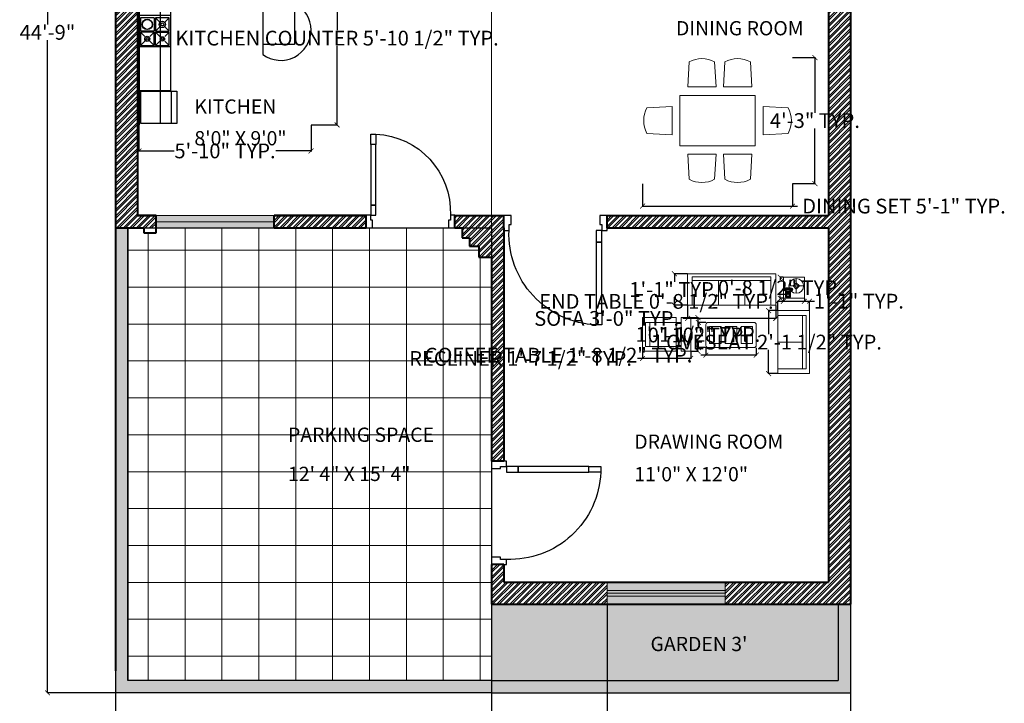
# Model space of a CAD drawing. Units: inches. Extents: x 528 to 2520, y -151 to 1354.
# Tile 29 of 41: x 2119 to 2520, y 357 to 635. Entities that reach past the tile are written whole.
import ezdxf

# ---------------------------------------------------------------- set-up
doc = ezdxf.new("R2010")
doc.units = ezdxf.units.IN
doc.header["$MEASUREMENT"] = 0
for name, color, linetype, lineweight in [('A-ANNO-DIMS', 2, 'Continuous', 18), ('A-AREA-IDEN', 7, 'Continuous', 18), ('A-Door', 150, 'Continuous', 25), ('A-ELEV-PROJ', 8, 'Continuous', 13), ('A-FLOR-CASE', 11, 'Continuous', 20), ('A-FLOR-PATT', 7, 'Continuous', 13), ('A-FURN', 8, 'Continuous', 18), ('A-SITE-EDGE', 7, 'Continuous', 25), ('A-SITE-PATT', 7, 'Continuous', 13), ('A-WALL-PATT', 6, 'Continuous', 13), ('walls', 7, 'Continuous', 40), ('WINDOWS', 2, 'Continuous', 20)]:
    doc.layers.add(name, color=color, linetype=linetype, lineweight=lineweight)
doc.layers.add('A-GLAZ-PATT', color=152, linetype='Continuous', lineweight=13, true_color=0x2776bb)
doc.layers.add('L-PLNT-PATT', color=85, linetype='Continuous', lineweight=13, true_color=0x58ba48)
for name, color, linetype in [('ESYA', 11, 'Continuous'), ('NT', 1, 'Continuous'), ('TEFRIS', 11, 'Continuous')]:
    doc.layers.add(name, color=color, linetype=linetype)
doc.styles.get("Standard").update_dxf_attribs({"font": 'arial.ttf'})
doc.dimstyles.get("Standard").update_dxf_attribs({"dimtxt": 6, "dimasz": 2, "dimexe": 0.18, "dimexo": 0.0625, "dimgap": 0.09, "dimtad": 0, "dimtih": 1, "dimtoh": 1, "dimdec": 1, "dimzin": 0, "dimdsep": 46, "dimlunit": 3, "dimtxsty": 'Standard', "dimblk": 'ARCHTICK', "dimcen": 0.09, "dimadec": 0, "dimazin": 0, "dimtfac": 1, "dimtdec": 1, "dimtofl": 0, "dimtmove": 0, "dimatfit": 3, "dimfxl": 1, "dimtolj": 1, "dimtzin": 0, "dimarcsym": 0})

# ---------------------------------------------------------------- blocks, each defined once
blk = doc.blocks.new('A$C7DB75F4D')
at = {"layer": 'A-Door'}
for points in [[(625, 740), (625, 660), (665, 660), (665, 740)], [(625, 180), (625, 660), (665, 660), (665, 180)], [(625, 100), (625, 180), (665, 180), (665, 100)], [(35, 100), (35, 60), (50, 60), (50, 50), (50, 0), (0, 0), (0, 100)], [(665, 100), (700, 100), (700, 0), (650, 0), (650, 50), (650, 60), (665, 60)]]:
    blk.add_lwpolyline(points, close=True, dxfattribs=at)
at = {"layer": 'NT'}
blk.add_arc((650, 125), 615.5, 92.32782, 182.32782, dxfattribs=at)
blk = doc.blocks.new('AR365L')
blk.add_line((0, 0.1), (0.61, 0.1))
blk.add_lwpolyline([(0, 0), (0, 0.68), (0.61, 0.68), (0.61, 0)], close=True)
blk = doc.blocks.new('FIRIN1')
at = {"layer": 'ESYA'}
for p, q in [((0.288, -0.05), (0.288, -0.301)), ((0.398, -0.132), (0.312, -0.05)), ((0.575, -0.05), (0.489, -0.132)), ((0.288, -0.301), (0.025, -0.301)), ((0.025, -0.324), (0.111, -0.406)), ((0.202, -0.406), (0.288, -0.324)), ((0.398, -0.219), (0.312, -0.301)), ((0.398, -0.406), (0.312, -0.324)), ((0.575, -0.301), (0.489, -0.219)), ((0.575, -0.324), (0.489, -0.406)), ((0.025, -0.575), (0.111, -0.493)), ((0.202, -0.493), (0.288, -0.575)), ((0.398, -0.493), (0.312, -0.575)), ((0.575, -0.575), (0.489, -0.493))]:
    blk.add_line(p, q, dxfattribs=at)
blk.add_lwpolyline([(0, 0), (0.6, 0), (0.6, -0.6), (0, -0.6)], close=True, dxfattribs=at)
for points in [[(0.288, -0.05), (0.025, -0.05), (0.025, -0.301)], [(0.312, -0.05), (0.312, -0.301), (0.575, -0.301)], [(0.575, -0.301), (0.575, -0.05), (0.312, -0.05)], [(0.288, -0.575), (0.288, -0.324), (0.025, -0.324)], [(0.025, -0.324), (0.025, -0.575)], [(0.312, -0.575), (0.312, -0.324), (0.575, -0.324)], [(0.312, -0.575), (0.575, -0.575), (0.575, -0.324)], [(0.025, -0.575), (0.288, -0.575)]]:
    blk.add_lwpolyline(points, dxfattribs=at)
for centre, radius in [((0.156, -0.175), 0.0986), ((0.156, -0.175), 0.0936), ((0.444, -0.175), 0.0597), ((0.444, -0.175), 0.0294), ((0.156, -0.45), 0.0492), ((0.156, -0.45), 0.0242), ((0.444, -0.45), 0.0398), ((0.444, -0.45), 0.0196)]:
    blk.add_circle(centre, radius, dxfattribs=at)
blk = doc.blocks.new('ncvn')
for p, q in [((77868.4, -4466.7), (77868.4, -4520.7)), ((77949.4, -4466.7), (77868.4, -4466.7)), ((77949.4, -4520.7), (77949.4, -4466.7))]:
    blk.add_line(p, q)
at = {"layer": 'TEFRIS'}
for p, q in [((77783.7, -4466.7), (77783.7, -4763.4)), ((77783.7, -4466.7), (78049.5, -4466.7)), ((77902, -4516.6), (77902, -4471.6)), ((78049.5, -4466.7), (78049.5, -4553.6)), ((77819.7, -4502.8), (77819.7, -4759.2)), ((77819.7, -4502.8), (78049.5, -4502.8)), ((77837.7, -4520.8), (77837.7, -4704.7)), ((77837.7, -4520.8), (77995.5, -4520.8)), ((77868.4, -4520.7), (77949.4, -4520.7)), ((77995.5, -4520.8), (77995.5, -4643)), ((78049.5, -4555), (78049.5, -4625.7)), ((78049.5, -4625.7), (77995.8, -4625.7)), ((77783.7, -4704.7), (77837.7, -4704.7))]:
    blk.add_line(p, q, dxfattribs=at)
for points in [[(77868.4, -4466.7), (77868.4, -4520.7), (77949.4, -4520.7), (77949.4, -4466.7)], [(77871.4, -4471.6), (77871.4, -4516.6), (77947, -4516.6), (77947, -4471.6)]]:
    blk.add_lwpolyline(points, close=True, dxfattribs=at)
for points in [[(77873.2, -4477.9), (77900.2, -4477.9, -1), (77900.2, -4479.7), (77873.2, -4479.7, -1), (77873.2, -4477.9)], [(77873.2, -4480.6), (77900.2, -4480.6, -1), (77900.2, -4482.4), (77873.2, -4482.4, -1), (77873.2, -4480.6)], [(77873.2, -4483.3), (77900.2, -4483.3, -1), (77900.2, -4485.1), (77873.2, -4485.1, -1), (77873.2, -4483.3)], [(77873.2, -4486), (77900.2, -4486, -1), (77900.2, -4487.8), (77873.2, -4487.8, -1), (77873.2, -4486)], [(77873.2, -4488.7), (77900.2, -4488.7, -1), (77900.2, -4490.5), (77873.2, -4490.5, -1), (77873.2, -4488.7)], [(77873.2, -4491.4), (77900.2, -4491.4, -1), (77900.2, -4493.2), (77873.2, -4493.2, -1), (77873.2, -4491.4)], [(77873.2, -4494.1), (77900.2, -4494.1, -1), (77900.2, -4495.9), (77873.2, -4495.9, -1), (77873.2, -4494.1)], [(77873.2, -4496.8), (77900.2, -4496.8, -1), (77900.2, -4498.6), (77873.2, -4498.6, -1), (77873.2, -4496.8)], [(77873.2, -4499.5), (77900.2, -4499.5, -1), (77900.2, -4501.3), (77873.2, -4501.3, -1), (77873.2, -4499.5)], [(77873.2, -4502.2), (77900.2, -4502.2, -1), (77900.2, -4504), (77873.2, -4504, -1), (77873.2, -4502.2)], [(77873.2, -4504.9), (77900.2, -4504.9, -1), (77900.2, -4506.7), (77873.2, -4506.7, -1), (77873.2, -4504.9)], [(77873.2, -4507.6), (77900.2, -4507.6, -1), (77900.2, -4509.4), (77873.2, -4509.4, -1), (77873.2, -4507.6)], [(77873.2, -4510.3), (77900.2, -4510.3, -1), (77900.2, -4512.1), (77873.2, -4512.1, -1), (77873.2, -4510.3)]]:
    blk.add_lwpolyline(points, format="xyb", dxfattribs=at)
for points in [[(77911.5, -4488.6), (77925, -4475, -1), (77926.3, -4476.3), (77912.7, -4489.8, -1)], [(77913.5, -4476.3), (77919.7, -4476.3, -0.563183), (77919.7, -4477.4), (77913.5, -4477.4, -1)], [(77935.3, -4476.3), (77929.2, -4476.3, 0.563183), (77929.2, -4477.4), (77935.3, -4477.4, 1)], [(77906, -4486.7), (77906, -4507.2, 0.414214), (77911.4, -4512.6), (77937.6, -4512.6, 0.414214), (77943, -4507.2), (77943, -4486.7, 0.414214), (77937.6, -4481.3), (77911.4, -4481.3, 0.414214)], [(77906.5, -4486.7), (77906.5, -4507.2, 0.414214), (77911.4, -4512.1), (77937.6, -4512.1, 0.414214), (77942.4, -4507.2), (77942.4, -4486.7, 0.414214), (77937.6, -4481.9), (77911.4, -4481.9, 0.414214)]]:
    blk.add_lwpolyline(points, format="xyb", close=True, dxfattribs=at)
for points in [[(77901.2, -4520.7), (77901.2, -4521.6), (77902.1, -4521.6), (77902.1, -4520.7)], [(77915.6, -4520.7), (77915.6, -4521.6), (77916.5, -4521.6), (77916.5, -4520.7)]]:
    blk.add_lwpolyline(points, dxfattribs=at)
for centre, radius in [((77913, -4488.3), 0.571), ((77924.9, -4498.5), 2.86)]:
    blk.add_circle(centre, radius, dxfattribs=at)
for centre, radius, start, end in [((77918.7, -4476.9), 1.71, 199.4712, 160.5288), ((77924.4, -4476.9), 1.71, 75, 195), ((77924.4, -4476.9), 1.71, 255, 15), ((77930.2, -4476.9), 1.71, 19.4712, 340.5288), ((78026.2, -4601.3), 51.8, 233.6588, 63.2671)]:
    blk.add_arc(centre, radius, start, end, dxfattribs=at)
at = {"layer": 'TEFRIS', "xscale": 90, "yscale": 90, "zscale": 90}
blk.add_blockref('FIRIN1', (77783.8, -4575.9), dxfattribs=at)
at = {"layer": 'TEFRIS', "xscale": 90, "yscale": 90, "zscale": 90, "rotation": 90}
blk.add_blockref('AR365L', (77848.2, -4760.9), dxfattribs=at)
blk = doc.blocks.new('RECLIN32')
for p, q in [((16, 0), (16, -32)), ((-11.5, -3), (11.5, -3)), ((-11.5, -32), (-11.5, -3)), ((-11.5, -7), (11.5, -7)), ((11.5, -3), (11.5, -32)), ((-11.5, -32), (-11.5, -37)), ((-10.5, -32), (-10.5, -37)), ((10.5, -32), (10.5, -37)), ((11.5, -32), (11.5, -37))]:
    blk.add_line(p, q)
blk.add_lwpolyline([(16, -32), (-16, -32), (-16, 0), (16, 0)])
blk.add_lwpolyline([(-16, -46), (-16, -37), (16, -37), (16, -46)], close=True)
blk = doc.blocks.new('LOVESET5')
for p, q in [((35.75, 0), (35.75, -30.00001)), ((-19.75, -3), (31.25, -3)), ((-19.75, -30.00001), (-19.75, -3)), ((-19.75, -6.5), (31.25, -6.5)), ((5.75, -6.5), (5.75, -30.00001)), ((31.25, -3), (31.25, -30.00001))]:
    blk.add_line(p, q)
for points in [[(35.75, -30.00001), (-24.25, -30.00001), (-24.25, 0), (24.25, 0)], [(24.25, 0), (35.75, 0)]]:
    blk.add_lwpolyline(points)
blk = doc.blocks.new('TBLEN20S')
blk.add_lwpolyline([(-10, -10), (-10, 10), (10, 10), (10, -10)], close=True)
blk = doc.blocks.new('LAMP')
for p, q in [((-1, 0), (-7, 0)), ((0, 3), (-3, 0)), ((-3, 0), (0, -3)), ((0, 7), (0, 1)), ((3, 0), (0, 3)), ((0, -3), (3, 0)), ((1, 0), (7, 0)), ((0, -1), (0, -7))]:
    blk.add_line(p, q)
for radius in [7, 1]:
    blk.add_circle((0, 0), radius)
blk = doc.blocks.new('SOFA7')
for p, q in [((-37.5, -3), (37.5, -3)), ((-37.5, -30), (-37.5, -3)), ((-37.5, -6.5), (37.5, -6.5)), ((-12.5, -6.5), (-12.5, -30)), ((12.5, -6.5), (12.5, -30)), ((37.5, -3), (37.5, -30))]:
    blk.add_line(p, q)
blk.add_lwpolyline([(-42, -30), (-42, 0), (42, 0), (42, -30)], close=True)
blk = doc.blocks.new('TBLWGLAS')
for p, q in [((-22, 0), (22, 0)), ((-24, -22), (-24, -2)), ((-20.5, -20), (-20.5, -4)), ((-20.5, -4), (-9.5, -4)), ((-9.5, -4), (-9.5, -20)), ((-5.5, -20), (-5.5, -4)), ((-5.5, -4), (5.5, -4)), ((5.5, -4), (5.5, -20)), ((9.5, -20), (9.5, -4)), ((9.5, -4), (20.5, -4)), ((20.5, -4), (20.5, -20)), ((24, -2), (24, -22)), ((22, -24), (-22, -24)), ((-9.5, -20), (-20.5, -20)), ((5.5, -20), (-5.5, -20)), ((20.5, -20), (9.5, -20))]:
    blk.add_line(p, q)
for centre, start, end in [((-22, -2), 90, 180), ((22, -2), 0, 90), ((-22, -22), 180, 270), ((22, -22), 270, 0)]:
    blk.add_arc(centre, 2, start, end)
blk = doc.blocks.new('PHONE')
for p, q in [((-3.99, 3.5), (-3.99, 2.5)), ((4.01, 3.5), (-3.99, 3.5)), ((-3.99, 2.5), (4.01, 2.5)), ((-2.49, -4.03), (-2.49, 1.92)), ((-2.02, 4.5), (2.02, 4.5)), ((-1.99, 1), (-1.99, -4)), ((2.01, 1), (-1.99, 1)), ((-1.49, 4), (-0.74, 4)), ((-1.49, 3.5), (-1.49, 4)), ((-1.49, 2), (-1.49, 2.5)), ((-0.74, 2), (-1.49, 2)), ((1.01, 0.5), (-0.99, 0.5)), ((-0.99, 0.5), (-0.99, -3.5)), ((-0.74, 4), (-0.74, 3.5)), ((-0.74, 2.5), (-0.74, 2)), ((0.76, 4), (0.76, 3.5)), ((1.51, 4), (0.76, 4)), ((0.76, 2.5), (0.76, 2)), ((0.76, 2), (1.51, 2)), ((1.01, -3.5), (1.01, 0.5)), ((1.51, 3.5), (1.51, 4)), ((1.51, 2), (1.51, 2.5)), ((2.01, -4), (2.01, 1)), ((2.51, 1.95), (2.51, -4.06)), ((4.01, 2.5), (4.01, 3.5)), ((2.04, -4.5), (-2.01, -4.5)), ((-1.99, -4), (2.01, -4)), ((-0.99, -3.5), (1.01, -3.5))]:
    blk.add_line(p, q)
for centre, radius, start, end in [((-3.24, 3), 1.27, 24.02748, 336.6167), ((-2.05, 4.06), 0.442, 81.8699, 188.1301), ((2.07, 4.06), 0.442, 351.8699, 98.1301), ((3.26, 3), 1.25, 205.0096, 154.8206), ((-2.05, -4.06), 0.442, 171.8699, 278.1301), ((2.07, -4.06), 0.442, 261.8699, 8.1301)]:
    blk.add_arc(centre, radius, start, end)
blk = doc.blocks.new('table-20')
at = {"color": 0, "linetype": 'ByBlock'}
for p, q in [((-1.052, 0.533), (-1.074, 0.134)), ((-0.646, 0.533), (-0.624, 0.134)), ((-0.484, 0.533), (-0.506, 0.134)), ((-0.078, 0.533), (-0.056, 0.134)), ((-1.2, 0), (0, 0)), ((-1.2, -0.8), (-1.2, 0)), ((-0.624, 0.134), (-1.074, 0.134)), ((-0.056, 0.134), (-0.506, 0.134)), ((0, -0.8), (0, 0)), ((-1.723, -0.197), (-1.324, -0.175)), ((-1.324, -0.625), (-1.324, -0.175)), ((0.124, -0.625), (0.124, -0.175)), ((0.523, -0.197), (0.124, -0.175)), ((-1.723, -0.603), (-1.324, -0.625)), ((0.523, -0.603), (0.124, -0.625)), ((-1.2, -0.8), (0, -0.8)), ((-0.624, -0.934), (-1.074, -0.934)), ((-1.052, -1.333), (-1.074, -0.934)), ((-0.646, -1.333), (-0.624, -0.934)), ((-0.484, -1.333), (-0.506, -0.934)), ((-0.056, -0.934), (-0.506, -0.934)), ((-0.078, -1.333), (-0.056, -0.934))]:
    blk.add_line(p, q, dxfattribs=at)
for centre, start, end in [((-0.849, 0.159), 61.4891, 118.5109), ((-0.281, 0.159), 61.4891, 118.5109), ((-1.349, -0.4), 151.4891, 208.5109), ((0.149, -0.4), 331.4891, 28.5109), ((-0.849, -0.959), 241.4891, 298.5109), ((-0.281, -0.959), 241.4891, 298.5109)]:
    blk.add_arc(centre, 0.425, start, end, dxfattribs=at)
blk = doc.blocks.new('WINDOW-48x5-PLAN')
for p, q in [((0, 5), (48, 5)), ((0, 2.5), (48, 2.5))]:
    blk.add_line(p, q)
blk.add_lwpolyline([(0, 5), (48, 5), (48, 0), (0, 0)], close=True)
blk = doc.blocks.new('WINDOW-48x9-PLAN')
for p, q in [((0, 5.63), (48, 5.63)), ((0, 4.5), (48, 4.5)), ((0, 3.37), (48, 3.37))]:
    blk.add_line(p, q)
blk.add_lwpolyline([(0, 9), (48, 9), (48, 0), (0, 0)], close=True)
blk = doc.blocks.new('TELEPHONE-KEYPAD')
for centre in [(0.05, 0.67), (0.07, 0.46), (0.09, 0.25), (0.1, 0.06), (0.26, 0.67), (0.27, 0.47), (0.27, 0.25), (0.29, 0.05), (0.48, 0.66), (0.48, 0.46), (0.49, 0.26), (0.5, 0.08)]:
    blk.add_circle(centre, 0.0493)
blk = doc.blocks.new('_ArchTick')
at = {"color": 0, "linetype": 'ByBlock', "const_width": 0.15}
blk.add_lwpolyline([(-0.5, -0.5), (0.5, 0.5)], dxfattribs=at)
blk = doc.blocks.new('*D60')
at = {"layer": 'A-ANNO-DIMS', "color": 0, "lineweight": -2, "transparency": 16777216}
for p, q in [((2237.62, 662.36), (2248.32, 662.36)), ((2248.14, 662.36), (2248.14, 630.29)), ((2248.14, 591.82), (2248.14, 623.9)), ((2237.62, 591.82), (2248.32, 591.82))]:
    blk.add_line(p, q, dxfattribs=at)
at = {"layer": 'Defpoints', "color": 0, "transparency": 16777216}
for p in [(2237.56, 662.36), (2248.14, 662.36), (2237.56, 591.82)]:
    blk.add_point(p, dxfattribs=at)
at = {"layer": 'A-ANNO-DIMS', "color": 0, "lineweight": -2, "transparency": 16777216, "xscale": 2, "yscale": 2, "zscale": 2}
for p, rotation in [((2248.14, 662.36), 90), ((2248.14, 591.82), 270)]:
    blk.add_blockref('_ArchTick', p, dxfattribs=dict(at, rotation=rotation))
at = {"layer": 'A-ANNO-DIMS', "color": 0, "transparency": 16777216, "insert": (2248.14, 627.09), "char_height": 6, "attachment_point": 5}
blk.add_mtext('\\A1;KITCHEN COUNTER 5\'-10 1/2" TYP.', dxfattribs=at)
blk = doc.blocks.new('*D61')
at = {"layer": 'A-ANNO-DIMS', "color": 0, "lineweight": -2, "transparency": 16777216}
for p, q in [((2167.57, 591.76), (2167.57, 581.06)), ((2237.56, 591.76), (2237.56, 581.06)), ((2167.57, 581.24), (2181.86, 581.24)), ((2237.56, 581.24), (2223.28, 581.24))]:
    blk.add_line(p, q, dxfattribs=at)
at = {"layer": 'Defpoints', "color": 0, "transparency": 16777216}
for p in [(2167.57, 591.82), (2237.56, 591.82), (2237.56, 581.24)]:
    blk.add_point(p, dxfattribs=at)
at = {"layer": 'A-ANNO-DIMS', "color": 0, "lineweight": -2, "transparency": 16777216, "xscale": 2, "yscale": 2, "zscale": 2, "rotation": 180}
blk.add_blockref('_ArchTick', (2167.57, 581.24), dxfattribs=at)
at = {"layer": 'A-ANNO-DIMS', "color": 0, "lineweight": -2, "transparency": 16777216, "xscale": 2, "yscale": 2, "zscale": 2}
blk.add_blockref('_ArchTick', (2237.56, 581.24), dxfattribs=at)
at = {"layer": 'A-ANNO-DIMS', "color": 0, "transparency": 16777216, "insert": (2202.57, 581.24), "char_height": 6, "attachment_point": 5}
blk.add_mtext('\\A1;5\'-10" TYP.', dxfattribs=at)
blk = doc.blocks.new('*D62')
at = {"layer": 'A-ANNO-DIMS', "color": 0, "lineweight": -2, "transparency": 16777216}
for p, q in [((2372.36, 496.88), (2370.36, 496.88)), ((2372.36, 499.76), (2372.36, 496.7)), ((2391.98, 496.88), (2372.36, 496.88)), ((2391.98, 499.76), (2391.98, 496.7))]:
    blk.add_line(p, q, dxfattribs=at)
at = {"layer": 'Defpoints', "color": 0, "transparency": 16777216}
for p in [(2372.36, 499.83), (2372.36, 496.88), (2391.98, 499.83)]:
    blk.add_point(p, dxfattribs=at)
at = {"layer": 'A-ANNO-DIMS', "color": 0, "lineweight": -2, "transparency": 16777216, "xscale": 2, "yscale": 2, "zscale": 2, "rotation": 180.0000000000005}
blk.add_blockref('_ArchTick', (2372.36, 496.88), dxfattribs=at)
at = {"layer": 'A-ANNO-DIMS', "color": 0, "lineweight": -2, "transparency": 16777216, "xscale": 2, "yscale": 2, "zscale": 2}
blk.add_blockref('_ArchTick', (2391.98, 496.88), dxfattribs=at)
at = {"layer": 'A-ANNO-DIMS', "color": 0, "transparency": 16777216, "insert": (2322.79, 496.88), "char_height": 6, "attachment_point": 5}
blk.add_mtext('\\A1;RECLINER 1\'-7 1/2" TYP.', dxfattribs=at)
blk = doc.blocks.new('*D63')
at = {"layer": 'A-ANNO-DIMS', "color": 0, "lineweight": -2, "transparency": 16777216}
for p, q in [((2392.04, 513.48), (2395.11, 513.48)), ((2394.93, 513.48), (2394.93, 509.85)), ((2394.93, 499.83), (2394.93, 503.46)), ((2392.04, 499.83), (2395.11, 499.83))]:
    blk.add_line(p, q, dxfattribs=at)
at = {"layer": 'Defpoints', "color": 0, "transparency": 16777216}
for p in [(2391.98, 513.48), (2391.98, 499.83), (2394.93, 499.83)]:
    blk.add_point(p, dxfattribs=at)
at = {"layer": 'A-ANNO-DIMS', "color": 0, "lineweight": -2, "transparency": 16777216, "xscale": 2, "yscale": 2, "zscale": 2}
for p, rotation in [((2394.93, 513.48), 90), ((2394.93, 499.83), 270)]:
    blk.add_blockref('_ArchTick', p, dxfattribs=dict(at, rotation=rotation))
at = {"layer": 'A-ANNO-DIMS', "color": 0, "transparency": 16777216, "insert": (2394.93, 506.65), "char_height": 6, "attachment_point": 5}
blk.add_mtext('\\A1;1\'-1 1/2" TYP.', dxfattribs=at)
blk = doc.blocks.new('*D64')
at = {"layer": 'A-ANNO-DIMS', "color": 0, "lineweight": -2, "transparency": 16777216}
for p, q in [((2427.44, 516.32), (2423.48, 516.32)), ((2423.66, 516.32), (2423.66, 506.71)), ((2423.66, 490.72), (2423.66, 500.32)), ((2427.44, 490.72), (2423.48, 490.72))]:
    blk.add_line(p, q, dxfattribs=at)
at = {"layer": 'Defpoints', "color": 0, "transparency": 16777216}
for p in [(2423.66, 516.32), (2427.5, 516.32), (2427.5, 490.72)]:
    blk.add_point(p, dxfattribs=at)
at = {"layer": 'A-ANNO-DIMS', "color": 0, "lineweight": -2, "transparency": 16777216, "xscale": 2, "yscale": 2, "zscale": 2}
for p, rotation in [((2423.66, 516.32), 90), ((2423.66, 490.72), 270)]:
    blk.add_blockref('_ArchTick', p, dxfattribs=dict(at, rotation=rotation))
at = {"layer": 'A-ANNO-DIMS', "color": 0, "transparency": 16777216, "insert": (2423.66, 503.52), "char_height": 6, "attachment_point": 5}
blk.add_mtext('\\A1;LOVESEAT 2\'-1 1/2" TYP.', dxfattribs=at)
blk = doc.blocks.new('*D65')
at = {"layer": 'A-ANNO-DIMS', "color": 0, "lineweight": -2, "transparency": 16777216}
for p, q in [((2427.5, 516.38), (2427.5, 520.34)), ((2427.5, 520.16), (2440.3, 520.16)), ((2440.3, 516.38), (2440.3, 520.34)), ((2440.3, 520.16), (2442.3, 520.16))]:
    blk.add_line(p, q, dxfattribs=at)
at = {"layer": 'Defpoints', "color": 0, "transparency": 16777216}
for p in [(2440.3, 520.16), (2427.5, 516.32), (2440.3, 516.32)]:
    blk.add_point(p, dxfattribs=at)
at = {"layer": 'A-ANNO-DIMS', "color": 0, "lineweight": -2, "transparency": 16777216, "xscale": 2, "yscale": 2, "zscale": 2, "rotation": 180}
blk.add_blockref('_ArchTick', (2427.5, 520.16), dxfattribs=at)
at = {"layer": 'A-ANNO-DIMS', "color": 0, "lineweight": -2, "transparency": 16777216, "xscale": 2, "yscale": 2, "zscale": 2}
blk.add_blockref('_ArchTick', (2440.3, 520.16), dxfattribs=at)
at = {"layer": 'A-ANNO-DIMS', "color": 0, "transparency": 16777216, "insert": (2460.39, 520.16), "char_height": 6, "attachment_point": 5}
blk.add_mtext('\\A1;1\'-1" TYP.', dxfattribs=at)
blk = doc.blocks.new('*D66')
at = {"layer": 'A-ANNO-DIMS', "color": 0, "lineweight": -2, "transparency": 16777216}
for p, q in [((2429.71, 521.3), (2429.71, 519.9)), ((2438.24, 521.3), (2438.24, 519.9)), ((2429.71, 520.08), (2427.71, 520.08)), ((2438.24, 520.08), (2429.71, 520.08))]:
    blk.add_line(p, q, dxfattribs=at)
at = {"layer": 'Defpoints', "color": 0, "transparency": 16777216}
for p in [(2429.71, 521.36), (2438.24, 521.36), (2429.71, 520.08)]:
    blk.add_point(p, dxfattribs=at)
at = {"layer": 'A-ANNO-DIMS', "color": 0, "lineweight": -2, "transparency": 16777216, "xscale": 2, "yscale": 2, "zscale": 2, "rotation": 180}
blk.add_blockref('_ArchTick', (2429.71, 520.08), dxfattribs=at)
at = {"layer": 'A-ANNO-DIMS', "color": 0, "lineweight": -2, "transparency": 16777216, "xscale": 2, "yscale": 2, "zscale": 2}
blk.add_blockref('_ArchTick', (2438.24, 520.08), dxfattribs=at)
at = {"layer": 'A-ANNO-DIMS', "color": 0, "transparency": 16777216, "insert": (2378.05, 520.08), "char_height": 6, "attachment_point": 5}
blk.add_mtext('\\A1;END TABLE 0\'-8 1/2" TYP.', dxfattribs=at)
blk = doc.blocks.new('*D67')
at = {"layer": 'A-ANNO-DIMS', "color": 0, "lineweight": -2, "transparency": 16777216}
for p, q in [((2429.65, 529.89), (2428.25, 529.89)), ((2428.43, 529.89), (2428.43, 528.82)), ((2429.65, 521.36), (2428.25, 521.36)), ((2428.43, 521.36), (2428.43, 522.43))]:
    blk.add_line(p, q, dxfattribs=at)
at = {"layer": 'Defpoints', "color": 0, "transparency": 16777216}
for p in [(2428.43, 529.89), (2429.71, 529.89), (2429.71, 521.36)]:
    blk.add_point(p, dxfattribs=at)
at = {"layer": 'A-ANNO-DIMS', "color": 0, "lineweight": -2, "transparency": 16777216, "xscale": 2, "yscale": 2, "zscale": 2}
for p, rotation in [((2428.43, 529.89), 90), ((2428.43, 521.36), 270)]:
    blk.add_blockref('_ArchTick', p, dxfattribs=dict(at, rotation=rotation))
at = {"layer": 'A-ANNO-DIMS', "color": 0, "transparency": 16777216, "insert": (2428.43, 525.62), "char_height": 6, "attachment_point": 5}
blk.add_mtext('\\A1;0\'-8 1/2" TYP.', dxfattribs=at)
blk = doc.blocks.new('*D70')
at = {"layer": 'A-ANNO-DIMS', "color": 0, "lineweight": -2, "transparency": 16777216}
for p, q in [((2390.73, 518.46), (2390.73, 512.96)), ((2426.57, 518.46), (2426.57, 512.96)), ((2390.73, 513.14), (2388.73, 513.14)), ((2426.57, 513.14), (2390.73, 513.14))]:
    blk.add_line(p, q, dxfattribs=at)
at = {"layer": 'Defpoints', "color": 0, "transparency": 16777216}
for p in [(2390.73, 518.52), (2426.57, 518.52), (2390.73, 513.14)]:
    blk.add_point(p, dxfattribs=at)
at = {"layer": 'A-ANNO-DIMS', "color": 0, "lineweight": -2, "transparency": 16777216, "xscale": 2, "yscale": 2, "zscale": 2, "rotation": 180}
blk.add_blockref('_ArchTick', (2390.73, 513.14), dxfattribs=at)
at = {"layer": 'A-ANNO-DIMS', "color": 0, "lineweight": -2, "transparency": 16777216, "xscale": 2, "yscale": 2, "zscale": 2}
blk.add_blockref('_ArchTick', (2426.57, 513.14), dxfattribs=at)
at = {"layer": 'A-ANNO-DIMS', "color": 0, "transparency": 16777216, "insert": (2357.79, 513.14), "char_height": 6, "attachment_point": 5}
blk.add_mtext('\\A1;SOFA 3\'-0" TYP.', dxfattribs=at)
blk = doc.blocks.new('*D71')
at = {"layer": 'A-ANNO-DIMS', "color": 0, "lineweight": -2, "transparency": 16777216}
for p, q in [((2390.66, 531.32), (2385.17, 531.32)), ((2385.35, 531.32), (2385.35, 528.02)), ((2385.35, 518.52), (2385.35, 521.82)), ((2390.66, 518.52), (2385.17, 518.52))]:
    blk.add_line(p, q, dxfattribs=at)
at = {"layer": 'Defpoints', "color": 0, "transparency": 16777216}
for p in [(2385.35, 531.32), (2390.73, 531.32), (2390.73, 518.52)]:
    blk.add_point(p, dxfattribs=at)
at = {"layer": 'A-ANNO-DIMS', "color": 0, "lineweight": -2, "transparency": 16777216, "xscale": 2, "yscale": 2, "zscale": 2}
for p, rotation in [((2385.35, 531.32), 90), ((2385.35, 518.52), 270)]:
    blk.add_blockref('_ArchTick', p, dxfattribs=dict(at, rotation=rotation))
at = {"layer": 'A-ANNO-DIMS', "color": 0, "transparency": 16777216, "insert": (2385.35, 524.92), "char_height": 6, "attachment_point": 5}
blk.add_mtext('\\A1;1\'-1" TYP.', dxfattribs=at)
blk = doc.blocks.new('*D72')
at = {"layer": 'A-ANNO-DIMS', "color": 0, "lineweight": -2, "transparency": 16777216}
for p, q in [((2398.17, 501.23), (2398.17, 498.04)), ((2418.65, 501.23), (2418.65, 498.04)), ((2398.17, 498.22), (2396.17, 498.22)), ((2418.65, 498.22), (2398.17, 498.22))]:
    blk.add_line(p, q, dxfattribs=at)
at = {"layer": 'Defpoints', "color": 0, "transparency": 16777216}
for p in [(2398.17, 501.29), (2418.65, 501.29), (2398.17, 498.22)]:
    blk.add_point(p, dxfattribs=at)
at = {"layer": 'A-ANNO-DIMS', "color": 0, "lineweight": -2, "transparency": 16777216, "xscale": 2, "yscale": 2, "zscale": 2, "rotation": 180}
blk.add_blockref('_ArchTick', (2398.17, 498.22), dxfattribs=at)
at = {"layer": 'A-ANNO-DIMS', "color": 0, "lineweight": -2, "transparency": 16777216, "xscale": 2, "yscale": 2, "zscale": 2}
blk.add_blockref('_ArchTick', (2418.65, 498.22), dxfattribs=at)
at = {"layer": 'A-ANNO-DIMS', "color": 0, "transparency": 16777216, "insert": (2338.23, 498.22), "char_height": 6, "attachment_point": 5}
blk.add_mtext('\\A1;COFFEE TABLE 1\'-8 1/2" TYP.', dxfattribs=at)
blk = doc.blocks.new('*D73')
at = {"layer": 'A-ANNO-DIMS', "color": 0, "lineweight": -2, "transparency": 16777216}
for p, q in [((2398.11, 511.53), (2394.92, 511.53)), ((2395.1, 511.53), (2395.1, 509.56)), ((2398.11, 501.29), (2394.92, 501.29)), ((2395.1, 501.29), (2395.1, 503.26))]:
    blk.add_line(p, q, dxfattribs=at)
at = {"layer": 'Defpoints', "color": 0, "transparency": 16777216}
for p in [(2395.1, 511.53), (2398.17, 511.53), (2398.17, 501.29)]:
    blk.add_point(p, dxfattribs=at)
at = {"layer": 'A-ANNO-DIMS', "color": 0, "lineweight": -2, "transparency": 16777216, "xscale": 2, "yscale": 2, "zscale": 2}
for p, rotation in [((2395.1, 511.53), 90), ((2395.1, 501.29), 270)]:
    blk.add_blockref('_ArchTick', p, dxfattribs=dict(at, rotation=rotation))
at = {"layer": 'A-ANNO-DIMS', "color": 0, "transparency": 16777216, "insert": (2395.1, 506.41), "char_height": 6, "attachment_point": 5}
blk.add_mtext('\\A1;0\'-10" TYP.', dxfattribs=at)
blk = doc.blocks.new('*D78')
at = {"layer": 'A-ANNO-DIMS', "color": 0, "lineweight": -2, "transparency": 16777216}
for p, q in [((2372.43, 567.89), (2372.43, 558.63)), ((2433.38, 567.89), (2433.38, 558.63)), ((2372.43, 558.81), (2433.38, 558.81)), ((2433.38, 558.81), (2435.38, 558.81))]:
    blk.add_line(p, q, dxfattribs=at)
at = {"layer": 'Defpoints', "color": 0, "transparency": 16777216}
for p in [(2372.43, 567.95), (2433.38, 567.95), (2433.38, 558.81)]:
    blk.add_point(p, dxfattribs=at)
at = {"layer": 'A-ANNO-DIMS', "color": 0, "lineweight": -2, "transparency": 16777216, "xscale": 2, "yscale": 2, "zscale": 2, "rotation": 180}
blk.add_blockref('_ArchTick', (2372.43, 558.81), dxfattribs=at)
at = {"layer": 'A-ANNO-DIMS', "color": 0, "lineweight": -2, "transparency": 16777216, "xscale": 2, "yscale": 2, "zscale": 2}
blk.add_blockref('_ArchTick', (2433.38, 558.81), dxfattribs=at)
at = {"layer": 'A-ANNO-DIMS', "color": 0, "transparency": 16777216, "insert": (2478.75, 558.81), "char_height": 6, "attachment_point": 5}
blk.add_mtext('\\A1;DINING SET 5\'-1" TYP.', dxfattribs=at)
blk = doc.blocks.new('*D79')
at = {"layer": 'A-ANNO-DIMS', "color": 0, "lineweight": -2, "transparency": 16777216}
for p, q in [((2433.44, 619.18), (2442.7, 619.18)), ((2442.52, 619.18), (2442.52, 596.72)), ((2442.52, 567.95), (2442.52, 590.41)), ((2433.44, 567.95), (2442.7, 567.95))]:
    blk.add_line(p, q, dxfattribs=at)
at = {"layer": 'Defpoints', "color": 0, "transparency": 16777216}
for p in [(2433.38, 619.18), (2442.52, 619.18), (2433.38, 567.95)]:
    blk.add_point(p, dxfattribs=at)
at = {"layer": 'A-ANNO-DIMS', "color": 0, "lineweight": -2, "transparency": 16777216, "xscale": 2, "yscale": 2, "zscale": 2}
for p, rotation in [((2442.52, 619.18), 90), ((2442.52, 567.95), 270)]:
    blk.add_blockref('_ArchTick', p, dxfattribs=dict(at, rotation=rotation))
at = {"layer": 'A-ANNO-DIMS', "color": 0, "transparency": 16777216, "insert": (2442.52, 593.57), "char_height": 6, "attachment_point": 5}
blk.add_mtext('\\A1;4\'-3" TYP.', dxfattribs=at)
blk = doc.blocks.new('*D94')
at = {"layer": 'A-ANNO-DIMS', "color": 0, "lineweight": -2, "transparency": 16777216}
for p, q in [((2158.01, 360.88), (2158.01, 333.11)), ((2457.01, 360.88), (2457.01, 333.11)), ((2158.01, 333.29), (2294.73, 333.29)), ((2457.01, 333.29), (2320.29, 333.29))]:
    blk.add_line(p, q, dxfattribs=at)
at = {"layer": 'Defpoints', "color": 0, "transparency": 16777216}
for p in [(2158.01, 360.94), (2457.01, 360.94), (2457.01, 333.29)]:
    blk.add_point(p, dxfattribs=at)
at = {"layer": 'A-ANNO-DIMS', "color": 0, "lineweight": -2, "transparency": 16777216, "xscale": 2, "yscale": 2, "zscale": 2, "rotation": 180}
blk.add_blockref('_ArchTick', (2158.01, 333.29), dxfattribs=at)
at = {"layer": 'A-ANNO-DIMS', "color": 0, "lineweight": -2, "transparency": 16777216, "xscale": 2, "yscale": 2, "zscale": 2}
blk.add_blockref('_ArchTick', (2457.01, 333.29), dxfattribs=at)
at = {"layer": 'A-ANNO-DIMS', "color": 0, "transparency": 16777216, "insert": (2307.51, 333.29), "char_height": 6, "attachment_point": 5}
blk.add_mtext('\\A1;24\'-11"', dxfattribs=at)
blk = doc.blocks.new('*D95')
at = {"layer": 'A-ANNO-DIMS', "color": 0, "lineweight": -2, "transparency": 16777216}
for p, q in [((2157.95, 897.94), (2130.18, 897.94)), ((2130.36, 897.94), (2130.36, 632.59)), ((2130.36, 360.94), (2130.36, 626.29)), ((2157.95, 360.94), (2130.18, 360.94))]:
    blk.add_line(p, q, dxfattribs=at)
at = {"layer": 'Defpoints', "color": 0, "transparency": 16777216}
for p in [(2130.36, 897.94), (2158.01, 897.94), (2158.01, 360.94)]:
    blk.add_point(p, dxfattribs=at)
at = {"layer": 'A-ANNO-DIMS', "color": 0, "lineweight": -2, "transparency": 16777216, "xscale": 2, "yscale": 2, "zscale": 2}
for p, rotation in [((2130.36, 897.94), 90), ((2130.36, 360.94), 270)]:
    blk.add_blockref('_ArchTick', p, dxfattribs=dict(at, rotation=rotation))
at = {"layer": 'A-ANNO-DIMS', "color": 0, "transparency": 16777216, "insert": (2130.36, 629.44), "char_height": 6, "attachment_point": 5}
blk.add_mtext('\\A1;44\'-9"', dxfattribs=at)
blk = doc.blocks.new('*D100')
at = {"layer": 'A-ANNO-DIMS', "color": 0, "lineweight": -2, "transparency": 16777216}
for p, q in [((2311.01, 396.88), (2311.01, 333.11)), ((2358.01, 396.88), (2358.01, 333.11)), ((2311.01, 333.29), (2324.12, 333.29)), ((2358.01, 333.29), (2344.91, 333.29))]:
    blk.add_line(p, q, dxfattribs=at)
at = {"layer": 'Defpoints', "color": 0, "transparency": 16777216}
for p in [(2311.01, 396.94), (2358.01, 396.94), (2358.01, 333.29)]:
    blk.add_point(p, dxfattribs=at)
at = {"layer": 'A-ANNO-DIMS', "color": 0, "lineweight": -2, "transparency": 16777216, "xscale": 2, "yscale": 2, "zscale": 2, "rotation": 180}
blk.add_blockref('_ArchTick', (2311.01, 333.29), dxfattribs=at)
at = {"layer": 'A-ANNO-DIMS', "color": 0, "lineweight": -2, "transparency": 16777216, "xscale": 2, "yscale": 2, "zscale": 2}
blk.add_blockref('_ArchTick', (2358.01, 333.29), dxfattribs=at)
at = {"layer": 'A-ANNO-DIMS', "color": 0, "transparency": 16777216, "insert": (2334.51, 333.29), "char_height": 6, "attachment_point": 5}
blk.add_mtext('\\A1;3\'-11"', dxfattribs=at)

msp = doc.modelspace()

# ---------------------------------------------------------------- hatches: boundary and pattern name
at = {"layer": 'A-FLOR-PATT', "transparency": 33554523}
h = msp.add_hatch(dxfattribs=at)
h.set_pattern_fill('NET', color=256, scale=120)
h.set_pattern_definition([(0, (1571.315, -419.164), (0, 15), []), (90, (1571.315, -419.164), (-15, 9e-16), [])])
h.paths.add_polyline_path([(2311.01, 538.08), (2305.75, 538.08), (2305.75, 542.51), (2302.05, 542.51), (2302.05, 545.95), (2299.01, 545.95), (2299.01, 549.94), (2174.56, 549.94), (2174.56, 547.94), (2169.56, 547.94), (2169.56, 549.94), (2163.01, 549.94), (2163.01, 365.94), (2311.01, 365.94)])
at = {"layer": 'A-GLAZ-PATT'}
h = msp.add_hatch(color=256, dxfattribs=at)
h.dxf.hatch_style = 1
h.paths.add_polyline_path([(2222.56, 554.94), (2174.56, 554.94), (2174.56, 552.44), (2222.56, 552.44)])
h.paths.add_polyline_path([(2222.56, 552.44), (2174.56, 552.44), (2174.56, 549.94), (2222.56, 549.94)])
h = msp.add_hatch(color=256, dxfattribs=at)
h.dxf.hatch_style = 1
h.paths.add_polyline_path([(2406.01, 405.94), (2358.01, 405.94), (2358.01, 402.57), (2406.01, 402.57)])
h.paths.add_polyline_path([(2406.01, 402.57), (2358.01, 402.57), (2358.01, 401.44), (2406.01, 401.44)])
h.paths.add_polyline_path([(2406.01, 401.44), (2358.01, 401.44), (2358.01, 400.31), (2406.01, 400.31)])
h.paths.add_polyline_path([(2406.01, 400.31), (2358.01, 400.31), (2358.01, 396.94), (2406.01, 396.94)])
at = {"layer": 'A-SITE-PATT'}
h = msp.add_hatch(color=256, dxfattribs=at)
h.dxf.hatch_style = 1
h.paths.add_polyline_path([(2457.01, 396.94), (2452.01, 396.94), (2452.01, 365.94), (2311.01, 365.94), (2163.01, 365.94), (2163.01, 549.94), (2158.01, 549.94), (2158.01, 369.94), (2158.01, 360.94), (2311.01, 360.94), (2457.01, 360.94)])
at = {"layer": 'A-WALL-PATT'}
h = msp.add_hatch(dxfattribs=at)
h.set_pattern_fill('ANSI32', color=256, scale=5)
h.set_pattern_definition([(45, (1571.3155, -419.1643), (-1.3258252, 1.3258252), []), (45, (1572.1993, -419.1643), (-1.3258252, 1.3258252), [])])
h.paths.add_polyline_path([(2167.01, 744.69), (2158.01, 744.69), (2158.01, 549.94), (2169.56, 549.94), (2174.56, 549.94), (2174.56, 554.94), (2167.01, 554.94), (2167.01, 662.94), (2263.01, 662.94), (2263.01, 667.94), (2263.01, 686.94), (2269.01, 686.94), (2269.01, 691.94), (2258.01, 691.94), (2258.01, 667.94), (2167.01, 667.94)])
h.paths.add_polyline_path([(2260.02, 554.94), (2222.56, 554.94), (2222.56, 549.94), (2260.02, 549.94)])
h.paths.add_polyline_path([(2457.01, 752.2), (2448.01, 752.2), (2448.01, 691.94), (2358.01, 691.94), (2358.01, 686.94), (2448.01, 686.94), (2448.01, 554.94), (2358.01, 554.94), (2358.01, 549.94), (2448.01, 549.94), (2448.01, 405.94), (2406.01, 405.94), (2406.01, 396.94), (2457.01, 396.94)])
h.paths.add_polyline_path([(2457.01, 897.94), (2447.97, 897.94), (2447.97, 888.94), (2448.01, 888.94), (2448.01, 828.94), (2394.01, 828.94), (2394.01, 823.94), (2448.01, 823.94), (2448.01, 800.2), (2457.01, 800.2)])
h.paths.add_polyline_path([(2423.97, 897.94), (2359.01, 897.94), (2359.01, 828.94), (2355.58, 828.94), (2355.58, 823.94), (2364.01, 823.94), (2364.01, 829.94), (2364.01, 888.94), (2423.97, 888.94)])
h.paths.add_polyline_path([(2256.01, 897.94), (2191.01, 897.94), (2191.01, 888.94), (2251.01, 888.94), (2251.01, 828.94), (2251.01, 823.94), (2256.01, 823.94), (2256.01, 829.08)])
h.paths.add_polyline_path([(2167.01, 888.94), (2167.01, 897.94), (2158.01, 897.94), (2158.01, 792.69), (2167.01, 792.69), (2167.01, 823.94), (2221.01, 823.94), (2221.01, 828.94), (2167.01, 828.94)])
h.paths.add_polyline_path([(2316.01, 549.94), (2316.01, 554.94), (2296.02, 554.94), (2296.02, 549.94), (2311.01, 549.94), (2311.01, 455.12), (2316.01, 455.12)])
h.paths.add_polyline_path([(2311.01, 549.94), (2299.01, 549.94), (2299.01, 545.95), (2302.05, 545.95), (2302.05, 542.51), (2305.75, 542.51), (2305.75, 538.08), (2311.01, 538.08)], flags=17)
h.paths.add_polyline_path([(2358.01, 405.94), (2316.01, 405.94), (2316.01, 413.12), (2311.01, 413.12), (2311.01, 396.94), (2358.01, 396.94)])
at = {"layer": 'L-PLNT-PATT', "transparency": 33554577}
h = msp.add_hatch(color=256, dxfattribs=at)
h.dxf.hatch_style = 1
h.paths.add_polyline_path([(2452.01, 396.94), (2311.01, 396.94), (2311.01, 365.94), (2452.01, 365.94)])
h.paths.add_polyline_path([(2374.14, 376.32), (2420.06, 376.32), (2420.06, 385.31), (2374.14, 385.31)], flags=24)

# ---------------------------------------------------------------- linework, layer by layer
at = {"layer": 'A-ELEV-PROJ'}
for p, q in [((2158.01, 360.94), (2158.01, 897.94)), ((2311.01, 360.94), (2311.01, 897.94)), ((2457.01, 360.94), (2457.01, 897.94))]:
    msp.add_line(p, q, dxfattribs=at)
at = {"layer": 'A-SITE-EDGE'}
for p, q in [((2163.01, 549.94), (2163.01, 365.94)), ((2311.01, 396.94), (2311.01, 365.94)), ((2452.01, 396.94), (2452.01, 365.94)), ((2457.01, 396.94), (2457.01, 360.94)), ((2158.01, 369.94), (2158.01, 360.94)), ((2311.01, 365.94), (2163.01, 365.94)), ((2311.01, 365.94), (2452.01, 365.94)), ((2311.01, 360.94), (2158.01, 360.94)), ((2311.01, 360.94), (2457.01, 360.94))]:
    msp.add_line(p, q, dxfattribs=at)
msp.add_lwpolyline([(2163.01, 549.94), (2311.01, 549.94), (2311.01, 365.94), (2163.01, 365.94)], close=True, dxfattribs=at)
at = {"layer": 'walls'}
for p, q in [((2158.01, 897.94), (2158.01, 369.94)), ((2457.01, 897.94), (2457.01, 396.94)), ((2448.01, 686.94), (2448.01, 554.94)), ((2167.01, 662.94), (2167.01, 554.94)), ((2167.01, 554.94), (2174.56, 554.94)), ((2174.56, 554.94), (2167.01, 554.94)), ((2174.56, 547.94), (2174.56, 554.94)), ((2222.56, 554.94), (2260.02, 554.94)), ((2260.02, 554.94), (2222.56, 554.94)), ((2222.56, 549.94), (2222.56, 554.94)), ((2260.02, 549.94), (2260.02, 554.94)), ((2296.02, 554.94), (2316.01, 554.94)), ((2296.02, 549.94), (2296.02, 554.94)), ((2316.01, 549.94), (2316.01, 554.94)), ((2358.01, 554.94), (2448.01, 554.94)), ((2358.01, 549.94), (2358.01, 554.94)), ((2158.01, 549.94), (2169.56, 549.94)), ((2169.56, 549.94), (2169.56, 547.94)), ((2222.56, 549.94), (2260.02, 549.94)), ((2296.02, 549.94), (2299.01, 549.94)), ((2299.01, 549.94), (2299.01, 545.95)), ((2316.01, 549.94), (2316.01, 455.12)), ((2358.01, 549.94), (2448.01, 549.94)), ((2448.01, 549.94), (2448.01, 405.94)), ((2169.56, 547.94), (2174.56, 547.94)), ((2299.01, 545.95), (2302.05, 545.95)), ((2302.05, 545.95), (2302.05, 542.51)), ((2302.05, 542.51), (2305.75, 542.51)), ((2305.75, 542.51), (2305.75, 538.08)), ((2305.75, 538.08), (2311.01, 538.08)), ((2311.01, 538.08), (2311.01, 455.12)), ((2316.01, 455.12), (2311.01, 455.12)), ((2311.01, 413.12), (2311.01, 396.94)), ((2316.01, 413.12), (2311.01, 413.12)), ((2316.01, 413.12), (2316.01, 405.94)), ((2316.01, 405.94), (2448.01, 405.94)), ((2311.01, 396.94), (2457.01, 396.94))]:
    msp.add_line(p, q, dxfattribs=at)

# ---------------------------------------------------------------- block references
at = {"layer": 'A-Door', "xscale": -0.0514539602427209, "yscale": 0.0514539602427209, "zscale": 0.0514539602427209}
msp.add_blockref('A$C7DB75F4D', (2296.04, 549.94), dxfattribs=at)
at = {"layer": 'A-Door', "xscale": -0.0600000000000059, "yscale": 0.0600000000000059, "zscale": 0.0600000000000059}
for p, rotation in [((2316.01, 554.94), 180), ((2311.01, 413.12), 270)]:
    msp.add_blockref('A$C7DB75F4D', p, dxfattribs=dict(at, rotation=rotation))
at = {"layer": 'A-FLOR-CASE', "xscale": 0.2377471155606993, "yscale": 0.2377471155606993, "zscale": 0.2377471155606993}
msp.add_blockref('ncvn', (-16325.27, 1724.3), dxfattribs=at)
at = {"layer": 'A-FURN', "xscale": 25.57841077690889, "yscale": 25.57841077690889, "zscale": 25.57841077690889}
msp.add_blockref('table-20', (2418.25, 603.8), dxfattribs=at)
at = {"layer": 'A-FURN', "extrusion": (0, 0, -1), "xscale": 0.4266539259093383, "yscale": 0.4266539259093383, "zscale": -0.426653925909338}
for name, p in [('SOFA7', (-2408.65, 531.32)), ('TBLEN20S', (-2433.98, 525.62)), ('LAMP', (-2434.93, 526.34)), ('PHONE', (-2431.57, 523.65)), ('TBLWGLAS', (-2408.41, 511.53))]:
    msp.add_blockref(name, p, dxfattribs=at)
at = {"layer": 'A-FURN'}
msp.add_blockref('TELEPHONE-KEYPAD', (2431.31, 522.92), dxfattribs=at)
at = {"layer": 'A-FURN', "extrusion": (0, 0, -1), "xscale": 0.4266539259093436, "yscale": 0.4266539259093436, "zscale": -0.426653925909338}
for name, p, rotation in [('RECLIN32', (-2372.36, 506.65), 269.9999999999994), ('LOVESET5', (-2440.3, 501.07), 89.99999999999947)]:
    msp.add_blockref(name, p, dxfattribs=dict(at, rotation=rotation))
at = {"layer": 'WINDOWS'}
for name, p in [('WINDOW-48x5-PLAN', (2174.56, 549.94)), ('WINDOW-48x9-PLAN', (2358.01, 396.94))]:
    msp.add_blockref(name, p, dxfattribs=at)

# ---------------------------------------------------------------- texts
at = {"layer": 'A-AREA-IDEN'}
for s, height, p in [('DINING ROOM', 5.7926, (2386.02, 628.22)), ('KITCHEN', 5.793, (2190.12, 596.38)), ('8\'0" X 9\'0"', 5.7926, (2190.12, 583.5)), ('PARKING SPACE', 5.7926, (2228.2, 462.97)), ('DRAWING ROOM', 5.7926, (2369.05, 460.16)), ('12\' 4" X 15\' 4"', 5.7926, (2228.2, 447.05)), ('11\'0" X 12\'0"', 5.7926, (2369.05, 446.94)), ("GARDEN 3'", 5.793, (2375.64, 377.92))]:
    msp.add_text(s, height=height, dxfattribs=at).set_placement(p)

# ---------------------------------------------------------------- dimensions: what is measured, and where the dimension line sits
at = {"layer": 'A-ANNO-DIMS'}
dim = msp.add_linear_dim(base=(2130.36, 897.94), p1=(2158.01, 360.94), p2=(2158.01, 897.94), angle=90, dimstyle='Standard', override={"dimdec": 1, "dimlfac": 1, "dimrnd": 0, "dimzin": 1, "dimdsep": 46, "dimlunit": 4, "dimfrac": 2}, dxfattribs=at)
dim.commit()
dim.dimension.update_dxf_attribs({"geometry": '*D95', "text_midpoint": (2130.36, 629.44)})
for base, p1, p2, angle, text, picture, middle in [((2248.14, 662.36), (2237.56, 591.82), (2237.56, 662.36), 90, 'KITCHEN COUNTER <> TYP.', '*D60', (2248.14, 627.09)), ((2442.52, 619.18), (2433.38, 567.95), (2433.38, 619.18), 90, '<> TYP.', '*D79', (2442.52, 593.57)), ((2429.71, 520.08), (2438.24, 521.36), (2429.71, 521.36), 180, 'END TABLE <> TYP.', '*D66', (2378.05, 520.08)), ((2428.43, 529.89), (2429.71, 521.36), (2429.71, 529.89), 90, '<> TYP.', '*D67', (2428.43, 525.62)), ((2385.35, 531.32), (2390.73, 518.52), (2390.73, 531.32), 90, '<> TYP.', '*D71', (2385.35, 524.92)), ((2440.3, 520.16), (2427.5, 516.32), (2440.3, 516.32), 0, '<> TYP.', '*D65', (2460.39, 520.16)), ((2390.73, 513.14), (2426.57, 518.52), (2390.73, 518.52), 180, 'SOFA <> TYP.', '*D70', (2357.79, 513.14)), ((2398.17, 498.22), (2418.65, 501.29), (2398.17, 501.29), 180, 'COFFEE TABLE <> TYP.', '*D72', (2338.23, 498.22)), ((2423.66, 516.32), (2427.5, 490.72), (2427.5, 516.32), 90, 'LOVESEAT <> TYP.', '*D64', (2423.66, 503.52)), ((2394.9255, 499.8272), (2391.9816, 513.4801), (2391.9816, 499.8272), 270, '<> TYP.', '*D63', (2394.9255, 506.6537)), ((2372.36, 496.88), (2391.98, 499.83), (2372.36, 499.83), 180, 'RECLINER <> TYP.', '*D62', (2322.79, 496.88)), ((2395.1, 511.53), (2398.17, 501.29), (2398.17, 511.53), 90, '<> TYP.', '*D73', (2395.1, 506.41))]:
    dim = msp.add_linear_dim(base=base, p1=p1, p2=p2, angle=angle, text=text, dimstyle='Standard', override={"dimdec": 1, "dimlfac": 1, "dimrnd": 0, "dimzin": 1, "dimdsep": 46, "dimlunit": 4, "dimfrac": 2}, dxfattribs=at)
    dim.commit()
    dim.dimension.update_dxf_attribs({"geometry": picture, "text_midpoint": middle})
for base, p1, p2, text, picture, middle in [((2237.56, 581.24), (2167.57, 591.82), (2237.56, 591.82), '<> TYP.', '*D61', (2202.57, 581.24)), ((2433.3781, 558.8115), (2372.4274, 567.9541), (2433.3781, 567.9541), 'DINING SET <> TYP.', '*D78', (2478.7532, 558.8115))]:
    dim = msp.add_linear_dim(base=base, p1=p1, p2=p2, text=text, dimstyle='Standard', override={"dimdec": 1, "dimlfac": 1, "dimrnd": 0, "dimzin": 1, "dimdsep": 46, "dimlunit": 4, "dimfrac": 2}, dxfattribs=at)
    dim.commit()
    dim.dimension.update_dxf_attribs({"geometry": picture, "text_midpoint": middle})
for base, p1, p2, picture, middle in [((2358.01, 333.29), (2311.01, 396.94), (2358.01, 396.94), '*D100', (2334.51, 333.29)), ((2457.01, 333.29), (2158.01, 360.94), (2457.01, 360.94), '*D94', (2307.51, 333.29))]:
    dim = msp.add_linear_dim(base=base, p1=p1, p2=p2, dimstyle='Standard', override={"dimdec": 1, "dimlfac": 1, "dimrnd": 0, "dimzin": 1, "dimdsep": 46, "dimlunit": 4, "dimfrac": 2}, dxfattribs=at)
    dim.commit()
    dim.dimension.update_dxf_attribs({"geometry": picture, "text_midpoint": middle})

doc.saveas('drawing.dxf')
